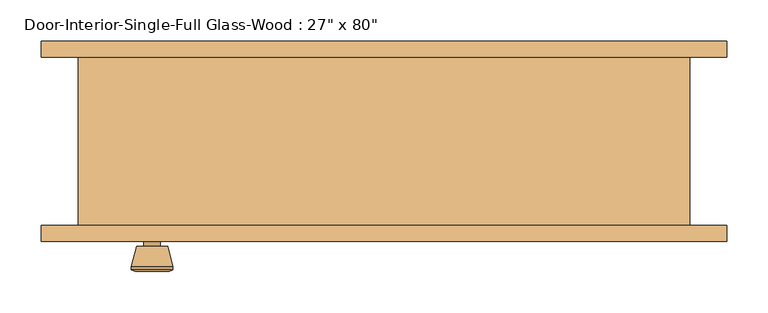
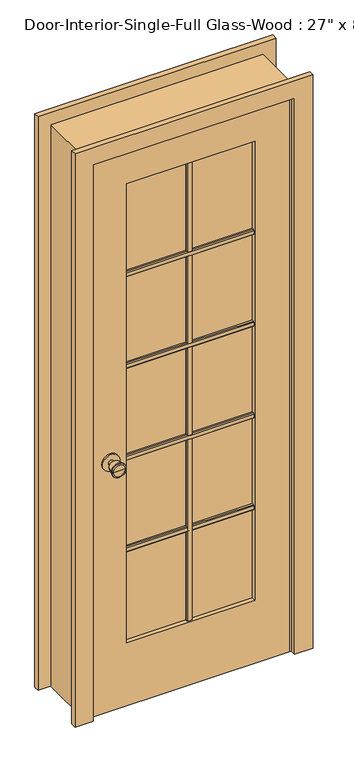
"""IFC4 building model written with IfcOpenShell, lengths in millimetres: door geometry."""

from ifc_helpers import new_model, si_unit, point, frame, frame_2d, origin, place, context, project, spatial, polyline, circle_curve, trimmed, segment, composite_curve, outline, extrude, faceted_brep, source, transform, mapped, element, save
from ifc_brep_helpers import plane_surface, cylinder_surface, revolved_surface, advanced_brep


def door_30d62acf(model_context):
    return source(origin(), model_context, "Body", "SolidModel", [
        extrude(outline(polyline([(-84.455, 1586.23), (-84.455, 1567.18), (-90.805, 1567.18), (-93.98, 1570.355), (-93.98, 1583.055), (-90.805, 1586.23), (-84.455, 1586.23)])), frame((-222.25, 0.0, 0.0), z_axis=(1.0, 0.0, 0.0), x_axis=(0.0, 1.0, 0.0)), (0.0, 0.0, 1.0), 444.5),
        extrude(outline(polyline([(-84.455, 1249.9975), (-84.455, 1230.9475), (-90.805, 1230.9475), (-93.98, 1234.1225), (-93.98, 1246.8225), (-90.805, 1249.9975), (-84.455, 1249.9975)])), frame((-222.25, 0.0, 0.0), z_axis=(1.0, 0.0, 0.0), x_axis=(0.0, 1.0, 0.0)), (0.0, 0.0, 1.0), 444.5),
        extrude(outline(polyline([(-84.455, 913.765), (-84.455, 894.715), (-90.805, 894.715), (-93.98, 897.89), (-93.98, 910.59), (-90.805, 913.765), (-84.455, 913.765)])), frame((-222.25, 0.0, 0.0), z_axis=(1.0, 0.0, 0.0), x_axis=(0.0, 1.0, 0.0)), (0.0, 0.0, 1.0), 444.5),
        extrude(outline(polyline([(-9.525, -84.455), (9.525, -84.455), (9.525, -90.805), (6.35, -93.98), (-6.35, -93.98), (-9.525, -90.805), (-9.525, -84.455)])), frame((0.0, 0.0, 231.775), z_axis=(0.0, 0.0, 1.0), x_axis=(1.0, 0.0, 0.0)), (0.0, 0.0, 1.0), 1681.1625),
        extrude(outline(polyline([(-84.455, 577.5325), (-84.455, 558.4825), (-90.805, 558.4825), (-93.98, 561.6575), (-93.98, 574.3575), (-90.805, 577.5325), (-84.455, 577.5325)])), frame((-222.25, 0.0, 0.0), z_axis=(1.0, 0.0, 0.0), x_axis=(0.0, 1.0, 0.0)), (0.0, 0.0, 1.0), 444.5),
        extrude(outline(polyline([(-77.47, 1586.23), (-71.12, 1586.23), (-67.945, 1583.055), (-67.945, 1570.355), (-71.12, 1567.18), (-77.47, 1567.18), (-77.47, 1586.23)])), frame((-222.25, 0.0, 0.0), z_axis=(1.0, 0.0, 0.0), x_axis=(0.0, 1.0, 0.0)), (0.0, 0.0, 1.0), 444.5),
        extrude(outline(polyline([(-77.47, 1249.9975), (-71.12, 1249.9975), (-67.945, 1246.8225), (-67.945, 1234.1225), (-71.12, 1230.9475), (-77.47, 1230.9475), (-77.47, 1249.9975)])), frame((-222.25, 0.0, 0.0), z_axis=(1.0, 0.0, 0.0), x_axis=(0.0, 1.0, 0.0)), (0.0, 0.0, 1.0), 444.5),
        extrude(outline(polyline([(-77.47, 913.765), (-71.12, 913.765), (-67.945, 910.59), (-67.945, 897.89), (-71.12, 894.715), (-77.47, 894.715), (-77.47, 913.765)])), frame((-222.25, 0.0, 0.0), z_axis=(1.0, 0.0, 0.0), x_axis=(0.0, 1.0, 0.0)), (0.0, 0.0, 1.0), 444.5),
        extrude(outline(polyline([(-9.525, -77.47), (-9.525, -71.12), (-6.35, -67.945), (6.35, -67.945), (9.525, -71.12), (9.525, -77.47), (-9.525, -77.47)])), frame((0.0, 0.0, 231.775), z_axis=(0.0, 0.0, 1.0), x_axis=(1.0, 0.0, 0.0)), (0.0, 0.0, 1.0), 1681.1625),
        extrude(outline(polyline([(-77.47, 577.5325), (-71.12, 577.5325), (-67.945, 574.3575), (-67.945, 561.6575), (-71.12, 558.4825), (-77.47, 558.4825), (-77.47, 577.5325)])), frame((-222.25, 0.0, 0.0), z_axis=(1.0, 0.0, 0.0), x_axis=(0.0, 1.0, 0.0)), (0.0, 0.0, 1.0), 444.5),
        advanced_brep(
        [(-279.4, -57.5, 914.4), (-289.4, -57.5, 914.4), (-269.4, -57.5, 914.4), (-258.9241324, -8.5, 914.4), (-299.8758676, -8.5, 914.4), (-279.4, -8.5, 914.4), (-254.4, -10.3278681, 914.4), (-304.4, -10.3278681, 914.4), (-254.4, -13.7915463, 914.4), (-304.4, -13.7915463, 914.4), (-260.763764, -38.5, 914.4), (-298.036236, -38.5, 914.4), (-269.4, -38.5, 914.4), (-289.4, -38.5, 914.4)],
        [
            (0, 1),
            (1, 2, circle_curve(frame((-279.4, -57.5, 914.4), z_axis=(0.0, -1.0, 0.0), x_axis=(-1.0, 0.0, 0.0)), 10.0)),
            (2, 0),
            (2, 1, circle_curve(frame((-279.4, -57.5, 914.4), z_axis=(0.0, -1.0, 0.0), x_axis=(-1.0, 0.0, 0.0)), 10.0)),
            (3, 4, circle_curve(frame((-279.4, -8.5, 914.4), z_axis=(0.0, 1.0, 0.0), x_axis=(-1.0, 0.0, 0.0)), 20.4758676)),
            (4, 5),
            (5, 3),
            (4, 3, circle_curve(frame((-279.4, -8.5, 914.4), z_axis=(0.0, 1.0, 0.0), x_axis=(-1.0, 0.0, 0.0)), 20.4758676)),
            (6, 7, circle_curve(frame((-279.4, -10.3278681, 914.4), z_axis=(0.0, 1.0, 0.0), x_axis=(-1.0, 0.0, 0.0)), 25.0)),
            (7, 4),
            (3, 6),
            (7, 6, circle_curve(frame((-279.4, -10.3278681, 914.4), z_axis=(0.0, 1.0, 0.0), x_axis=(-1.0, 0.0, 0.0)), 25.0)),
            (8, 9, circle_curve(frame((-279.4, -13.7915463, 914.4), z_axis=(0.0, 1.0, 0.0), x_axis=(-1.0, 0.0, 0.0)), 25.0)),
            (9, 7),
            (6, 8),
            (9, 8, circle_curve(frame((-279.4, -13.7915463, 914.4), z_axis=(0.0, 1.0, 0.0), x_axis=(-1.0, 0.0, 0.0)), 25.0)),
            (10, 11, circle_curve(frame((-279.4, -38.5, 914.4), z_axis=(0.0, 1.0, 0.0), x_axis=(-1.0, 0.0, 0.0)), 18.636236)),
            (11, 9),
            (8, 10),
            (11, 10, circle_curve(frame((-279.4, -38.5, 914.4), z_axis=(0.0, 1.0, 0.0), x_axis=(-1.0, 0.0, 0.0)), 18.636236)),
            (12, 13, circle_curve(frame((-279.4, -38.5, 914.4), z_axis=(0.0, 1.0, 0.0), x_axis=(-1.0, 0.0, 0.0)), 10.0)),
            (13, 11),
            (10, 12),
            (13, 12, circle_curve(frame((-279.4, -38.5, 914.4), z_axis=(0.0, 1.0, 0.0), x_axis=(-1.0, 0.0, 0.0)), 10.0)),
            (1, 13),
            (12, 2),
        ],
        [
            plane_surface(frame((-279.4, -57.5, 914.4), z_axis=(0.0, -1.0, 0.0), x_axis=(-1.0, 0.0, 0.0))),
            plane_surface(frame((-279.4, -8.5, 914.4), z_axis=(0.0, 1.0, 0.0), x_axis=(-1.0, 0.0, 0.0))),
            revolved_surface(polyline([(-299.8758676, -8.5, 914.4), (-304.4, -10.3278681, 914.4)]), (-279.4, -57.5, 914.4), (0.0, -1.0, 0.0)),
            cylinder_surface(frame((-279.4, -57.5, 914.4), z_axis=(0.0, -1.0, 0.0), x_axis=(-1.0, 0.0, 0.0)), 25.0),
            revolved_surface(polyline([(-304.4, -13.7915463, 914.4), (-298.036236, -38.5, 914.4)]), (-279.4, -57.5, 914.4), (0.0, -1.0, 0.0)),
            plane_surface(frame((-279.4, -38.5, 914.4), z_axis=(0.0, -1.0, 0.0), x_axis=(-1.0, 0.0, 0.0))),
            cylinder_surface(frame((-279.4, -57.5, 914.4), z_axis=(0.0, -1.0, 0.0), x_axis=(-1.0, 0.0, 0.0)), 10.0),
        ],
        [
            (0, [[1, 2, 3]]),
            (0, [[-3, 4, -1]]),
            (1, [[5, 6, 7]]),
            (1, [[8, -7, -6]]),
            (2, [[9, 10, -5, 11]]),
            (2, [[12, -11, -8, -10]]),
            (3, [[13, 14, -9, 15]]),
            (3, [[16, -15, -12, -14]]),
            (4, [[17, 18, -13, 19]]),
            (4, [[20, -19, -16, -18]]),
            (5, [[21, 22, -17, 23]]),
            (5, [[24, -23, -20, -22]]),
            (6, [[-2, 25, -21, 26]]),
            (6, [[-4, -26, -24, -25]]),
        ],
    ),
        extrude(outline(composite_curve([segment(trimmed(circle_curve(frame_2d((914.4, -279.4)), 30.0), [point((914.4, -309.4))], [point((914.4, -249.4))], False, "CARTESIAN"), True, "CONTINUOUS"), segment(trimmed(circle_curve(frame_2d((914.4, -279.4)), 30.0), [point((914.4, -249.4))], [point((914.4, -309.4))], False, "CARTESIAN"), True, "CONTINUOUS")], self_intersect=False)), frame((0.0, -63.5, 0.0), z_axis=(0.0, 1.0, 0.0), x_axis=(0.0, 0.0, 1.0)), (0.0, 0.0, 1.0), 6.0),
        advanced_brep(
        [(-279.4, -104.425, 914.4), (-269.4, -104.425, 914.4), (-289.4, -104.425, 914.4), (-258.9241324, -153.425, 914.4), (-279.4, -153.425, 914.4), (-299.8758676, -153.425, 914.4), (-254.4, -151.5971319, 914.4), (-304.4, -151.5971319, 914.4), (-254.4, -148.1334537, 914.4), (-304.4, -148.1334537, 914.4), (-260.763764, -123.425, 914.4), (-298.036236, -123.425, 914.4), (-269.4, -123.425, 914.4), (-289.4, -123.425, 914.4)],
        [
            (0, 1),
            (1, 2, circle_curve(frame((-279.4, -104.425, 914.4), z_axis=(0.0, 1.0, 0.0), x_axis=(-1.0, 0.0, 0.0)), 10.0)),
            (2, 0),
            (2, 1, circle_curve(frame((-279.4, -104.425, 914.4), z_axis=(0.0, 1.0, 0.0), x_axis=(-1.0, 0.0, 0.0)), 10.0)),
            (3, 4),
            (4, 5),
            (5, 3, circle_curve(frame((-279.4, -153.425, 914.4), z_axis=(0.0, -1.0, 0.0), x_axis=(-1.0, 0.0, 0.0)), 20.4758676)),
            (3, 5, circle_curve(frame((-279.4, -153.425, 914.4), z_axis=(0.0, -1.0, 0.0), x_axis=(-1.0, 0.0, 0.0)), 20.4758676)),
            (6, 3),
            (5, 7),
            (7, 6, circle_curve(frame((-279.4, -151.5971319, 914.4), z_axis=(0.0, -1.0, 0.0), x_axis=(-1.0, 0.0, 0.0)), 25.0)),
            (6, 7, circle_curve(frame((-279.4, -151.5971319, 914.4), z_axis=(0.0, -1.0, 0.0), x_axis=(-1.0, 0.0, 0.0)), 25.0)),
            (8, 6),
            (7, 9),
            (9, 8, circle_curve(frame((-279.4, -148.1334537, 914.4), z_axis=(0.0, -1.0, 0.0), x_axis=(-1.0, 0.0, 0.0)), 25.0)),
            (8, 9, circle_curve(frame((-279.4, -148.1334537, 914.4), z_axis=(0.0, -1.0, 0.0), x_axis=(-1.0, 0.0, 0.0)), 25.0)),
            (10, 8),
            (9, 11),
            (11, 10, circle_curve(frame((-279.4, -123.425, 914.4), z_axis=(0.0, -1.0, 0.0), x_axis=(-1.0, 0.0, 0.0)), 18.636236)),
            (10, 11, circle_curve(frame((-279.4, -123.425, 914.4), z_axis=(0.0, -1.0, 0.0), x_axis=(-1.0, 0.0, 0.0)), 18.636236)),
            (12, 10),
            (11, 13),
            (13, 12, circle_curve(frame((-279.4, -123.425, 914.4), z_axis=(0.0, -1.0, 0.0), x_axis=(-1.0, 0.0, 0.0)), 10.0)),
            (12, 13, circle_curve(frame((-279.4, -123.425, 914.4), z_axis=(0.0, -1.0, 0.0), x_axis=(-1.0, 0.0, 0.0)), 10.0)),
            (1, 12),
            (13, 2),
        ],
        [
            plane_surface(frame((-279.4, -104.425, 914.4), z_axis=(0.0, 1.0, 0.0), x_axis=(-1.0, 0.0, 0.0))),
            plane_surface(frame((-279.4, -153.425, 914.4), z_axis=(0.0, -1.0, 0.0), x_axis=(-1.0, 0.0, 0.0))),
            revolved_surface(polyline([(-299.8758676, -153.425, 914.4), (-304.4, -151.5971319, 914.4)]), (-279.4, -104.425, 914.4), (0.0, 1.0, 0.0)),
            cylinder_surface(frame((-279.4, -104.425, 914.4), z_axis=(0.0, 1.0, 0.0), x_axis=(-1.0, 0.0, 0.0)), 25.0),
            revolved_surface(polyline([(-304.4, -148.1334537, 914.4), (-298.036236, -123.425, 914.4)]), (-279.4, -104.425, 914.4), (0.0, 1.0, 0.0)),
            plane_surface(frame((-279.4, -123.425, 914.4), z_axis=(0.0, 1.0, 0.0), x_axis=(-1.0, 0.0, 0.0))),
            cylinder_surface(frame((-279.4, -104.425, 914.4), z_axis=(0.0, 1.0, 0.0), x_axis=(-1.0, 0.0, 0.0)), 10.0),
        ],
        [
            (0, [[1, 2, 3]]),
            (0, [[-3, 4, -1]]),
            (1, [[5, 6, 7]]),
            (1, [[-6, -5, 8]]),
            (2, [[9, -7, 10, 11]]),
            (2, [[-10, -8, -9, 12]]),
            (3, [[13, -11, 14, 15]]),
            (3, [[-14, -12, -13, 16]]),
            (4, [[17, -15, 18, 19]]),
            (4, [[-18, -16, -17, 20]]),
            (5, [[21, -19, 22, 23]]),
            (5, [[-22, -20, -21, 24]]),
            (6, [[25, -23, 26, -2]]),
            (6, [[-26, -24, -25, -4]]),
        ],
    ),
        extrude(outline(composite_curve([segment(trimmed(circle_curve(frame_2d((914.4, -279.4)), 30.0), [point((914.4, -309.4))], [point((914.4, -249.4))], False, "CARTESIAN"), True, "CONTINUOUS"), segment(trimmed(circle_curve(frame_2d((914.4, -279.4)), 30.0), [point((914.4, -249.4))], [point((914.4, -309.4))], False, "CARTESIAN"), True, "CONTINUOUS")], self_intersect=False)), frame((0.0, -104.425, 0.0), z_axis=(0.0, 1.0, 0.0), x_axis=(0.0, 0.0, 1.0)), (0.0, 0.0, 1.0), 6.0),
        extrude(outline(polyline([(2032.0, -342.9), (0.0, -342.9), (0.0, 342.9), (2032.0, 342.9), (2032.0, -342.9)]), holes=[polyline([(1912.9375, -222.25), (1912.9375, 222.25), (231.775, 222.25), (231.775, -222.25), (1912.9375, -222.25)])]), frame((0.0, -98.425, 0.0), z_axis=(0.0, 1.0, 0.0), x_axis=(0.0, 0.0, 1.0)), (0.0, 0.0, 1.0), 34.925),
        faceted_brep([(368.3, -98.425, 0.0), (342.9, -98.425, 0.0), (342.9, -63.5, 0.0), (330.2, -63.5, 0.0), (330.2, -28.575, 0.0), (342.9, -28.575, 0.0), (342.9, 104.775, 0.0), (368.3, 104.775, 0.0), (368.3, 104.775, 2057.4), (368.3, -98.425, 2057.4), (342.9, 104.775, 2032.0), (-342.9, 104.775, 2032.0), (-342.9, 104.775, 0.0), (-368.3, 104.775, 0.0), (-368.3, 104.775, 2057.4), (342.9, -28.575, 2032.0), (330.2, -28.575, 2019.3), (-330.2, -28.575, 2019.3), (-330.2, -28.575, 0.0), (-342.9, -28.575, 0.0), (-342.9, -28.575, 2032.0), (330.2, -63.5, 2019.3), (342.9, -63.5, 2032.0), (-342.9, -63.5, 2032.0), (-342.9, -63.5, 0.0), (-330.2, -63.5, 0.0), (-330.2, -63.5, 2019.3), (342.9, -98.425, 2032.0), (-368.3, -98.425, 2057.4), (-368.3, -98.425, 0.0), (-342.9, -98.425, 0.0), (-342.9, -98.425, 2032.0)], [[[0, 1, 2, 3, 4, 5, 6, 7]], [[7, 8, 9, 0]], [[6, 10, 11, 12, 13, 14, 8, 7]], [[5, 15, 10, 6]], [[4, 16, 17, 18, 19, 20, 15, 5]], [[3, 21, 16, 4]], [[2, 22, 23, 24, 25, 26, 21, 3]], [[1, 27, 22, 2]], [[0, 9, 28, 29, 30, 31, 27, 1]], [[8, 14, 28, 9]], [[15, 20, 11, 10]], [[21, 26, 17, 16]], [[27, 31, 23, 22]], [[29, 13, 12, 19, 18, 25, 24, 30]], [[14, 13, 29, 28]], [[20, 19, 12, 11]], [[26, 25, 18, 17]], [[31, 30, 24, 23]]]),
        extrude(outline(polyline([(222.25, -77.47), (222.25, -84.455), (-222.25, -84.455), (-222.25, -77.47), (222.25, -77.47)])), frame((0.0, 0.0, 231.775), z_axis=(0.0, 0.0, 1.0), x_axis=(1.0, 0.0, 0.0)), (0.0, 0.0, 1.0), 1681.1625),
        extrude(outline(polyline([(0.0, 412.75), (2101.85, 412.75), (2101.85, -412.75), (0.0, -412.75), (0.0, -349.25), (2038.35, -349.25), (2038.35, 349.25), (0.0, 349.25), (0.0, 412.75)])), frame((0.0, 104.775, 0.0), z_axis=(0.0, 1.0, 0.0), x_axis=(0.0, 0.0, 1.0)), (0.0, 0.0, 1.0), 19.05),
        extrude(outline(polyline([(0.0, 412.75), (2101.85, 412.75), (2101.85, -412.75), (0.0, -412.75), (0.0, -349.25), (2038.35, -349.25), (2038.35, 349.25), (0.0, 349.25), (0.0, 412.75)])), frame((0.0, -117.475, 0.0), z_axis=(0.0, 1.0, 0.0), x_axis=(0.0, 0.0, 1.0)), (0.0, 0.0, 1.0), 19.05),
    ])


if __name__ == "__main__":
    model = new_model("IFC4")
    model_context = context("Model", 3, world=origin())
    ifc_project = project(units=[si_unit("LENGTHUNIT", "METRE", prefix="MILLI")], contexts=[model_context])
    site = spatial("IfcSite", under=ifc_project)
    building = spatial("IfcBuilding", under=site)
    placement = place(None, origin())
    door_shape = door_30d62acf(model_context)
    element("IfcDoor", 1, ObjectType="Door-Interior-Single-Full Glass-Wood : 27\" x 80\"", at=placement, inside=building, context=model_context, shape_type="MappedRepresentation", body=[
        mapped(door_shape, transform((0.0, 0.0, 0.0), x_axis=(1.0, 0.0, 0.0), y_axis=(0.0, 1.0, 0.0), z_axis=(0.0, 0.0, 1.0))),
    ])
    save(model, "model.ifc")

# Revit data of these elements
# Type "Door-Interior-Single-Full Glass-Wood : 27\" x 80\""
#   Type Mark = "10"
#   Assembly Code = "C1020300"
#   Analytic Construction = "Wood frame with single clear glass"
#   Top Rail = 0' - 4 11/16"
#   Thickness = 0' - 1 3/8"
#   Thermal Resistance (R) = 1.0102 (h·ft²·°F)/BTU
#   Swing Angle [instance default] = 90.00°
#   Stiles = 0' - 4 3/4"
#   Rough Width = 2' - 5"
#   Rough Height = 6' - 9"
#   Height = 6' - 8"
#   Width = 2' - 3"
#   Heat Transfer Coefficient (U) = 0.9900 BTU/(h·ft²·°F)
#   Bottom Rail = 0' - 9 1/8"
#   Show Grill [instance default] = yes
#   Trim Material = Cherry
#   Panel Material = Cherry
#   Frame Material = Cherry
#   Door Handle Material = Aluminum
#   Visual Light Transmittance = 0
#   Solar Heat Gain Coefficient = 0
#   Wall Closure = (empty or 0)
#   Function = (empty or 0)
# Element 1 (IfcDoor, "Door-Interior-Single-Full Glass-Wood : 27\" x 80\"")
#   Materials on its faces: "Cherry", "Aluminum", "Glass"
# Materials
#   "Cherry": class "Wood", colour RGB 226 177 128, transparency 0, Description = "Prunus Serotina", Cost = 0
#   "Aluminum": class "Metal", colour RGB 247 247 247, transparency 0, Description = "Aluminum 6061", Cost = 0
#   "Glass": class "Glass", colour RGB 0 128 192, transparency 0.75, Description = "Soda Lime Glass", Cost = 0
